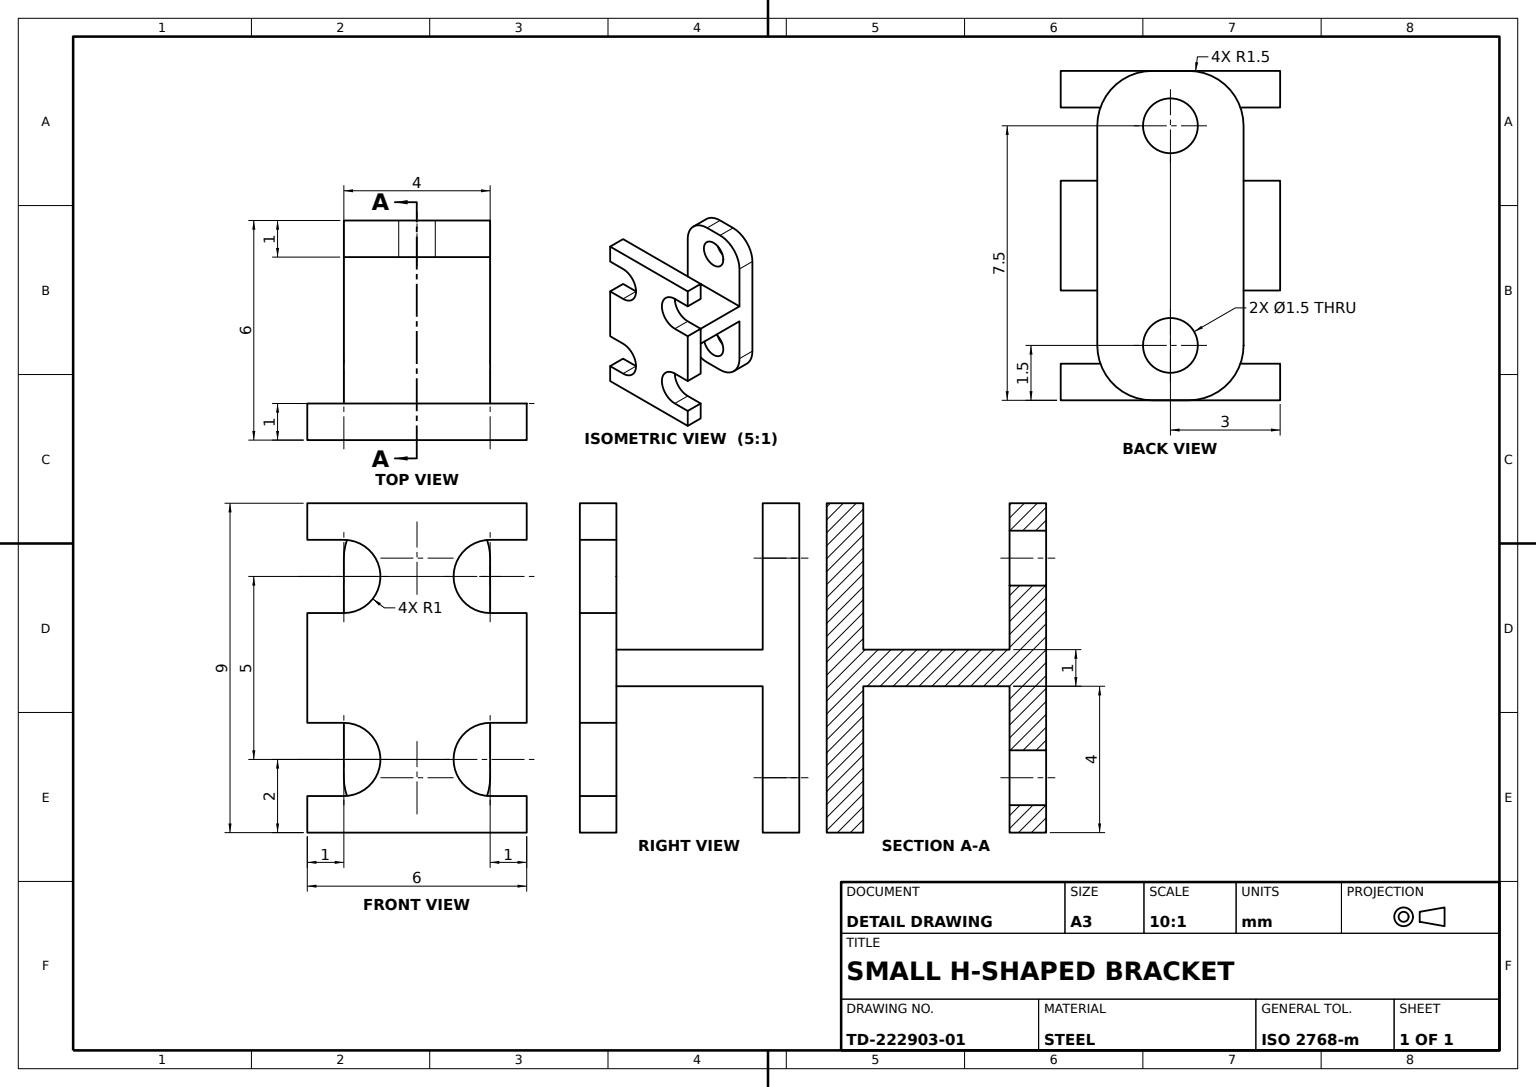
from build123d import *

# Parameters (mm, degrees)
BASE_PLATE_DEPTH         = 1
STANDOFF_WEB_SKETCH_W    = 4
STANDOFF_WEB_SKETCH_H    = 1
STANDOFF_WEB_4MM_DEPTH   = 4
FORK_LUG_SKETCH_W        = 4
FORK_LUG_SKETCH_H        = 9
FORK_LUG_DEPTH           = 1
LUG_END_FILLETS_R1_5_R   = 1.5
LUG_PIN_HOLES_SKETCH_R   = 0.75
LUG_PIN_HOLES_SKETCH_R_2 = 0.749568333
LUG_PIN_HOLES_DEPTH      = 1


with BuildPart() as part:
    # Base Plate Sketch → Base Plate (new body)
    with BuildSketch(Plane.XY):
        with BuildLine():
            Line((0, 0), (6, 0))
            Line((6, 0), (6, 1))
            Line((6, 1), (5, 1))
            ThreePointArc((5, 1), (4, 2), (5, 3))
            Line((5, 3), (6, 3))
            Line((6, 3), (6, 6))
            Line((6, 6), (5, 6))
            ThreePointArc((5, 6), (4, 7), (5, 8))
            Line((5, 8), (6, 8))
            Line((6, 8), (6, 9))
            Line((6, 9), (0, 9))
            Line((0, 9), (0, 8))
            Line((0, 8), (1, 8))
            ThreePointArc((1, 8), (2, 7), (1, 6))
            Line((1, 6), (0, 6))
            Line((0, 6), (0, 3))
            Line((0, 3), (1, 3))
            ThreePointArc((1, 3), (2, 2), (1, 1))
            Line((1, 1), (0, 1))
            Line((0, 1), (0, 0))
        make_face()
    extrude(amount=BASE_PLATE_DEPTH)

    # Standoff Web Sketch → Standoff Web 4mm (add)
    with BuildSketch(Plane(origin=(0, 0, 0), x_dir=(-1, 0, 0), z_dir=(0, 0, -1))):
        with Locations((-3, 4.5)):
            Rectangle(STANDOFF_WEB_SKETCH_W, STANDOFF_WEB_SKETCH_H)
    extrude(amount=STANDOFF_WEB_4MM_DEPTH)

    # Fork Lug Sketch → Fork Lug (add)
    with BuildSketch(Plane(origin=(0, 0, -4), x_dir=(-1, 0, 0), z_dir=(0, 0, -1))):
        with Locations((-3, 4.5)):
            Rectangle(FORK_LUG_SKETCH_W, FORK_LUG_SKETCH_H)
    extrude(amount=FORK_LUG_DEPTH)

    # Lug End Fillets R1.5
    lug_end_fillets_r1_5_edges = [part.edges().sort_by_distance(p)[0] for p in [
        (1, 0, -4.5),
        (1, 9, -4.5),
        (5, 9, -4.5),
        (5, 0, -4.5),
    ]]
    fillet(lug_end_fillets_r1_5_edges, radius=LUG_END_FILLETS_R1_5_R)

    # Lug Pin Holes Sketch → Lug Pin Holes (cut)
    with BuildSketch(Plane(origin=(0, 0, -5), x_dir=(-1, 0, 0), z_dir=(0, 0, -1))):
        with Locations((-3, 7.5)):
            Circle(LUG_PIN_HOLES_SKETCH_R)
        with Locations((-3, 1.5)):
            Circle(LUG_PIN_HOLES_SKETCH_R_2)
    extrude(amount=-LUG_PIN_HOLES_DEPTH, mode=Mode.SUBTRACT)


solid = part.part
